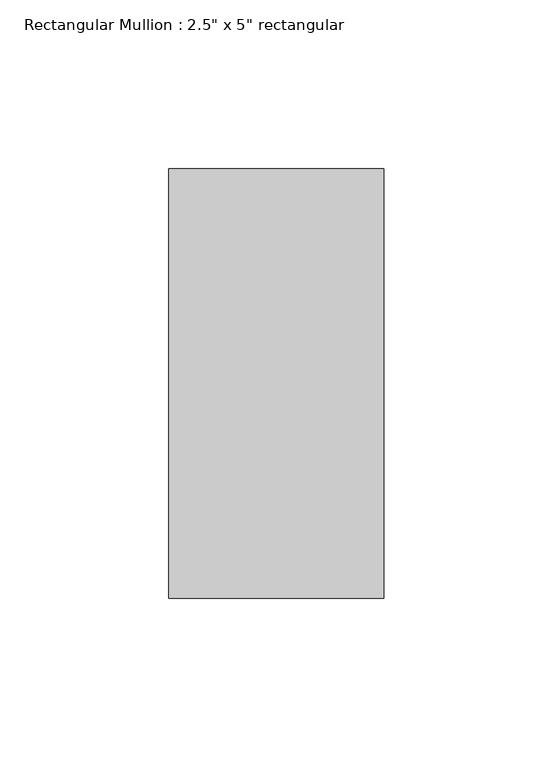
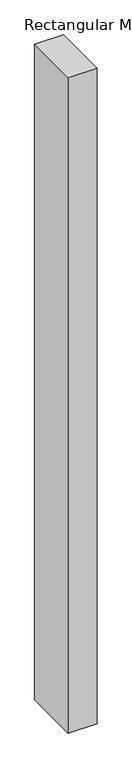
"""IFC4 building model written with IfcOpenShell, lengths in millimetres: member geometry."""

from ifc_helpers import new_model, si_unit, frame, origin, place, context, project, spatial, polyline, outline, extrude, source, transform, mapped, element, save


def member_4491d118(model_context):
    return source(origin(), model_context, "Body", "SweptSolid", [
        extrude(outline(polyline([(0.0, 63.5), (0.0, -63.5), (-63.5, -63.5), (-63.5, 63.5), (0.0, 63.5)])), frame((0.0, 0.0, -1524.0), z_axis=(0.0, 0.0, 1.0), x_axis=(1.0, 0.0, 0.0)), (0.0, 0.0, 1.0), 1524.0),
    ])


if __name__ == "__main__":
    model = new_model("IFC4")
    model_context = context("Model", 3, world=origin())
    ifc_project = project(units=[si_unit("LENGTHUNIT", "METRE", prefix="MILLI")], contexts=[model_context])
    site = spatial("IfcSite", under=ifc_project)
    building = spatial("IfcBuilding", under=site)
    placement = place(None, origin())
    member_shape = member_4491d118(model_context)
    element("IfcMember", 1, ObjectType="Rectangular Mullion : 2.5\" x 5\" rectangular", at=placement, inside=building, context=model_context, shape_type="MappedRepresentation", body=[
        mapped(member_shape, transform((0.0, 0.0, 0.0), x_axis=(1.0, 0.0, 0.0), y_axis=(0.0, 1.0, 0.0), z_axis=(0.0, 0.0, 1.0))),
    ])
    save(model, "model.ifc")

# Revit data of these elements
# Type "Rectangular Mullion : 2.5\" x 5\" rectangular"
#   built-in parameter 1007304 = 0.416667 (stored number, unit not read)
#   built-in parameter 1007301 = 0.104167 (stored number, unit not read)
#   built-in parameter 1007300 = 0.104167 (stored number, unit not read)
# Element 1 (IfcMember, "Rectangular Mullion : 2.5\" x 5\" rectangular")
#   Materials on its faces: "metal black"
# Materials
#   "metal black": class "Generic", colour RGB 120 120 120, transparency 0, Cost = 0
